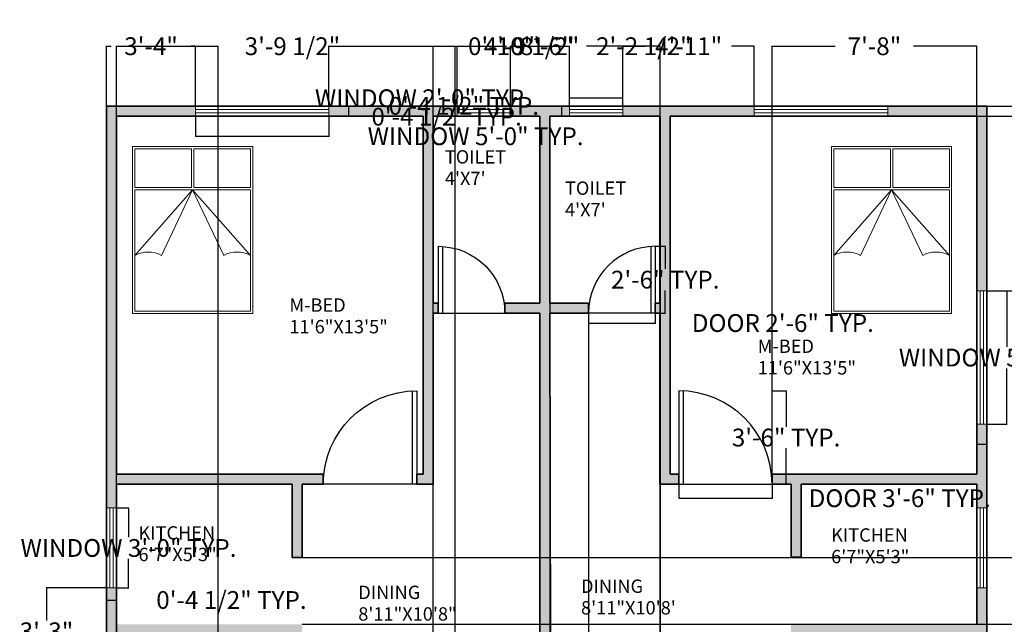
# Model space of a CAD drawing. Units: inches. Extents: x -27 to 662, y -19 to 539.
# Tile 3 of 4: x -18 to 425, y 267 to 539. Entities that reach past the tile are written whole.
import ezdxf

# ---------------------------------------------------------------- set-up
doc = ezdxf.new("R2010")
doc.units = ezdxf.units.IN
doc.header["$MEASUREMENT"] = 0
for name, color, linetype, lineweight in [('A-ANNO-DIMS', 2, 'Continuous', 18), ('A-AREA-IDEN', 230, 'Continuous', 18), ('A-DOOR', 6, 'Continuous', 25), ('A-FURN', 240, 'Continuous', 18), ('A-GLAZ', 240, 'Continuous', 18), ('A-WALL', 4, 'Continuous', 35)]:
    doc.layers.add(name, color=color, linetype=linetype, lineweight=lineweight)
doc.layers.add('A-WALL-PATT', color=2, linetype='Continuous', lineweight=13, true_color=0xf1eb1f)
doc.styles.get("Standard").update_dxf_attribs({"font": 'italic8.shx'})
doc.dimstyles.get("Standard").update_dxf_attribs({"dimtxt": 8, "dimasz": 0.18, "dimexe": 0.18, "dimexo": 0.0625, "dimgap": 0.09, "dimtad": 0, "dimtih": 1, "dimtoh": 1, "dimzin": 0, "dimdsep": 46, "dimlunit": 3, "dimtxsty": 'Standard', "dimcen": 0.09, "dimclrt": 4, "dimadec": 0, "dimazin": 0, "dimtfac": 1, "dimtofl": 0, "dimtmove": 0, "dimatfit": 3, "dimfxl": 1, "dimtolj": 1, "dimtzin": 0, "dimarcsym": 0})

# ---------------------------------------------------------------- blocks, each defined once
blk = doc.blocks.new('*D2')
at = {"layer": 'A-ANNO-DIMS', "color": 0, "lineweight": -2, "transparency": 16777216}
for p, q in [((391.54, 495.42), (467.74, 495.42)), ((467.56, 495.24), (467.56, 262.52)), ((467.56, 20.1), (467.56, 252.82)), ((391.54, 19.92), (467.74, 19.92))]:
    blk.add_line(p, q, dxfattribs=at)
at = {"layer": 'A-ANNO-DIMS', "color": 0, "transparency": 16777216}
for points in [[(467.53, 495.24), (467.59, 495.24), (467.56, 495.42)], [(467.53, 20.1), (467.59, 20.1), (467.56, 19.92)]]:
    blk.add_solid(points, dxfattribs=at)
at = {"layer": 'Defpoints', "color": 0, "transparency": 16777216}
for p in [(391.48, 495.42), (467.56, 495.42), (391.48, 19.92)]:
    blk.add_point(p, dxfattribs=at)
at = {"layer": 'A-ANNO-DIMS', "color": 0, "transparency": 16777216, "insert": (467.56, 257.67), "char_height": 8, "attachment_point": 5}
blk.add_mtext('\\A1;39\'-7.50"', dxfattribs=at)
blk = doc.blocks.new('BED-DOUBLE-54x75')
for p, q in [((26.5, 56.54), (26.5, 74)), ((27.5, 56.54), (27.5, 74)), ((1, 56.54), (26.5, 56.54)), ((1, 55.54), (53, 55.54)), ((27, 55.54), (1, 26.04)), ((13, 26.04), (27, 55.54)), ((27, 55.54), (53, 26.04)), ((41, 26.04), (27, 55.54)), ((27.5, 56.54), (53, 56.54))]:
    blk.add_line(p, q)
blk.add_lwpolyline([(0, 75), (54, 75), (54, 0), (0, 0)], close=True)
for points in [[(1, 56.54), (1, 74), (26.5, 74)], [(27.5, 74), (53, 74), (53, 56.54)], [(53, 55.54), (53, 1), (1, 1), (1, 55.54)]]:
    blk.add_lwpolyline(points)
for centre in [(7, 14.92), (47, 14.92)]:
    blk.add_arc(centre, 12.64, 61.656, 118.344)
blk = doc.blocks.new('DOOR-SWING-30IN')
for p, q in [((28, 29.93), (28, 0)), ((30, 30), (30, 0)), ((30, 0), (0, 0))]:
    blk.add_line(p, q)
blk.add_arc((30, 0), 30, 90, 180)
blk = doc.blocks.new('DOOR-SWING-42IN')
for p, q in [((0, 42), (0, 0)), ((2, 41.95), (2, 0)), ((0, 0), (42, 0))]:
    blk.add_line(p, q)
blk.add_arc((0, 0), 42, 0, 90)
blk = doc.blocks.new('WIN-60IN')
for p, q in [((0, 4.5), (0, 0)), ((60, 4.5), (0, 4.5)), ((60, 0), (60, 4.5)), ((0, 3), (60, 3)), ((0, 1.5), (60, 1.5)), ((0, 0), (60, 0))]:
    blk.add_line(p, q)
blk = doc.blocks.new('WIN-60IN-B')
for p, q in [((0, 0), (0, 60)), ((0, 60), (4.5, 60)), ((1.5, 0), (1.5, 60)), ((3, 0), (3, 60)), ((4.5, 60), (4.5, 0)), ((4.5, 0), (0, 0)), ((4.5, 0), (2.25, 0))]:
    blk.add_line(p, q)
blk = doc.blocks.new('WIN-36IN')
for p, q in [((0, 36), (4.5, 36)), ((0, 0), (0, 36)), ((0, 36), (2.25, 36)), ((1.5, 36), (1.5, 0)), ((3, 36), (3, 0)), ((4.5, 36), (4.5, 0)), ((4.5, 0), (0, 0))]:
    blk.add_line(p, q)
blk = doc.blocks.new('WIN-24IN')
for p, q in [((0, 4.5), (0, 0)), ((24, 4.5), (0, 4.5)), ((24, 0), (24, 4.5)), ((0, 3), (24, 3)), ((0, 1.5), (24, 1.5)), ((0, 0), (24, 0))]:
    blk.add_line(p, q)
blk = doc.blocks.new('*D14')
at = {"layer": 'A-ANNO-DIMS', "color": 0, "lineweight": -2, "transparency": 16777216}
for p, q in [((238.14, 406.86), (238.14, 402.24)), ((268.14, 406.86), (268.14, 402.24)), ((238.32, 402.42), (267.96, 402.42)), ((268.14, 402.42), (268.32, 402.42))]:
    blk.add_line(p, q, dxfattribs=at)
at = {"layer": 'A-ANNO-DIMS', "color": 0, "transparency": 16777216}
for points in [[(238.32, 402.45), (238.32, 402.39), (238.14, 402.42)], [(267.96, 402.45), (267.96, 402.39), (268.14, 402.42)]]:
    blk.add_solid(points, dxfattribs=at)
at = {"layer": 'Defpoints', "color": 0, "transparency": 16777216}
for p in [(238.14, 406.92), (268.14, 406.92), (268.14, 402.42)]:
    blk.add_point(p, dxfattribs=at)
at = {"layer": 'A-ANNO-DIMS', "color": 4, "transparency": 16777216, "insert": (325.55, 402.42), "char_height": 8, "attachment_point": 5}
blk.add_mtext('\\A1;DOOR 2\'-6" TYP.', dxfattribs=at)
blk = doc.blocks.new('*D15')
at = {"layer": 'A-ANNO-DIMS', "color": 0, "lineweight": -2, "transparency": 16777216}
for p, q in [((268.2, 436.92), (272.82, 436.92)), ((272.64, 436.74), (272.64, 426.77)), ((272.64, 407.1), (272.64, 417.07)), ((268.2, 406.92), (272.82, 406.92))]:
    blk.add_line(p, q, dxfattribs=at)
at = {"layer": 'A-ANNO-DIMS', "color": 0, "transparency": 16777216}
for points in [[(272.61, 436.74), (272.67, 436.74), (272.64, 436.92)], [(272.61, 407.1), (272.67, 407.1), (272.64, 406.92)]]:
    blk.add_solid(points, dxfattribs=at)
at = {"layer": 'Defpoints', "color": 0, "transparency": 16777216}
for p in [(268.14, 436.92), (272.64, 436.92), (268.14, 406.92)]:
    blk.add_point(p, dxfattribs=at)
at = {"layer": 'A-ANNO-DIMS', "color": 4, "transparency": 16777216, "insert": (272.64, 421.92), "char_height": 8, "attachment_point": 5}
blk.add_mtext('\\A1;2\'-6" TYP.', dxfattribs=at)
blk = doc.blocks.new('*D16')
at = {"layer": 'A-ANNO-DIMS', "color": 0, "lineweight": -2, "transparency": 16777216}
for p, q in [((278.72, 329.86), (278.72, 323.44)), ((320.72, 329.86), (320.72, 323.44)), ((278.9, 323.62), (320.54, 323.62)), ((320.72, 323.62), (320.9, 323.62))]:
    blk.add_line(p, q, dxfattribs=at)
at = {"layer": 'A-ANNO-DIMS', "color": 0, "transparency": 16777216}
for points in [[(278.9, 323.65), (278.9, 323.59), (278.72, 323.62)], [(320.54, 323.65), (320.54, 323.59), (320.72, 323.62)]]:
    blk.add_solid(points, dxfattribs=at)
at = {"layer": 'Defpoints', "color": 0, "transparency": 16777216}
for p in [(278.72, 329.92), (320.72, 329.92), (320.72, 323.62)]:
    blk.add_point(p, dxfattribs=at)
at = {"layer": 'A-ANNO-DIMS', "color": 4, "transparency": 16777216, "insert": (378.13, 323.62), "char_height": 8, "attachment_point": 5}
blk.add_mtext('\\A1;DOOR 3\'-6" TYP.', dxfattribs=at)
blk = doc.blocks.new('*D17')
at = {"layer": 'A-ANNO-DIMS', "color": 0, "lineweight": -2, "transparency": 16777216}
for p, q in [((320.78, 371.92), (327.2, 371.92)), ((327.02, 371.74), (327.02, 355.77)), ((327.02, 330.1), (327.02, 346.07)), ((320.78, 329.92), (327.2, 329.92))]:
    blk.add_line(p, q, dxfattribs=at)
at = {"layer": 'A-ANNO-DIMS', "color": 0, "transparency": 16777216}
for points in [[(326.99, 371.74), (327.05, 371.74), (327.02, 371.92)], [(326.99, 330.1), (327.05, 330.1), (327.02, 329.92)]]:
    blk.add_solid(points, dxfattribs=at)
at = {"layer": 'Defpoints', "color": 0, "transparency": 16777216}
for p in [(320.72, 371.92), (327.02, 371.92), (320.72, 329.92)]:
    blk.add_point(p, dxfattribs=at)
at = {"layer": 'A-ANNO-DIMS', "color": 4, "transparency": 16777216, "insert": (327.02, 350.92), "char_height": 8, "attachment_point": 5}
blk.add_mtext('\\A1;3\'-6" TYP.', dxfattribs=at)
blk = doc.blocks.new('*D20')
at = {"layer": 'A-ANNO-DIMS', "color": 0, "lineweight": -2, "transparency": 16777216}
for p, q in [((61.34, 495.36), (61.34, 486.24)), ((121.34, 495.36), (121.34, 486.24)), ((61.52, 486.42), (121.16, 486.42)), ((121.34, 486.42), (121.52, 486.42))]:
    blk.add_line(p, q, dxfattribs=at)
at = {"layer": 'A-ANNO-DIMS', "color": 0, "transparency": 16777216}
for points in [[(61.52, 486.45), (61.52, 486.39), (61.34, 486.42)], [(121.16, 486.45), (121.16, 486.39), (121.34, 486.42)]]:
    blk.add_solid(points, dxfattribs=at)
at = {"layer": 'Defpoints', "color": 0, "transparency": 16777216}
for p in [(61.34, 495.42), (121.34, 495.42), (121.34, 486.42)]:
    blk.add_point(p, dxfattribs=at)
at = {"layer": 'A-ANNO-DIMS', "color": 4, "transparency": 16777216, "insert": (187.33, 486.42), "char_height": 8, "attachment_point": 5}
blk.add_mtext('\\A1;WINDOW 5\'-0" TYP.', dxfattribs=at)
blk = doc.blocks.new('*D21')
at = {"layer": 'A-ANNO-DIMS', "color": 0, "lineweight": -2, "transparency": 16777216}
for p, q in [((121.4, 499.92), (130.52, 499.92)), ((130.34, 499.92), (130.34, 500.1)), ((130.34, 500.1), (130.52, 500.1)), ((130.34, 495.6), (130.34, 499.74)), ((121.4, 495.42), (130.52, 495.42))]:
    blk.add_line(p, q, dxfattribs=at)
at = {"layer": 'A-ANNO-DIMS', "color": 0, "transparency": 16777216}
for points in [[(130.31, 499.74), (130.37, 499.74), (130.34, 499.92)], [(130.31, 495.6), (130.37, 495.6), (130.34, 495.42)]]:
    blk.add_solid(points, dxfattribs=at)
at = {"layer": 'Defpoints', "color": 0, "transparency": 16777216}
for p in [(121.34, 499.92), (130.34, 499.92), (121.34, 495.42)]:
    blk.add_point(p, dxfattribs=at)
at = {"layer": 'A-ANNO-DIMS', "color": 4, "transparency": 16777216, "insert": (182.04, 500.1), "char_height": 8, "attachment_point": 5}
blk.add_mtext('\\A1;0\'-4 1/2" TYP.', dxfattribs=at)
blk = doc.blocks.new('*D22')
at = {"layer": 'A-ANNO-DIMS', "color": 0, "lineweight": -2, "transparency": 16777216}
for p, q in [((417.35, 416.88), (426.47, 416.88)), ((426.29, 416.7), (426.29, 391.73)), ((426.29, 357.06), (426.29, 382.03)), ((417.35, 356.88), (426.47, 356.88))]:
    blk.add_line(p, q, dxfattribs=at)
at = {"layer": 'A-ANNO-DIMS', "color": 0, "transparency": 16777216}
for points in [[(426.26, 416.7), (426.32, 416.7), (426.29, 416.88)], [(426.26, 357.06), (426.32, 357.06), (426.29, 356.88)]]:
    blk.add_solid(points, dxfattribs=at)
at = {"layer": 'Defpoints', "color": 0, "transparency": 16777216}
for p in [(417.29, 416.88), (426.29, 416.88), (417.29, 356.88)]:
    blk.add_point(p, dxfattribs=at)
at = {"layer": 'A-ANNO-DIMS', "color": 4, "transparency": 16777216, "insert": (426.29, 386.88), "char_height": 8, "attachment_point": 5}
blk.add_mtext('\\A1;WINDOW 5\'-0" TYP.', dxfattribs=at)
blk = doc.blocks.new('*D23')
at = {"layer": 'A-ANNO-DIMS', "color": 0, "lineweight": -2, "transparency": 16777216}
for p, q in [((412.79, 356.82), (412.79, 347.7)), ((417.29, 356.82), (417.29, 347.7)), ((412.97, 347.88), (417.11, 347.88)), ((417.29, 347.88), (417.47, 347.88))]:
    blk.add_line(p, q, dxfattribs=at)
at = {"layer": 'A-ANNO-DIMS', "color": 0, "transparency": 16777216}
for points in [[(412.97, 347.91), (412.97, 347.85), (412.79, 347.88)], [(417.11, 347.91), (417.11, 347.85), (417.29, 347.88)]]:
    blk.add_solid(points, dxfattribs=at)
at = {"layer": 'Defpoints', "color": 0, "transparency": 16777216}
for p in [(412.79, 356.88), (417.29, 356.88), (417.29, 347.88)]:
    blk.add_point(p, dxfattribs=at)
at = {"layer": 'A-ANNO-DIMS', "color": 4, "transparency": 16777216, "insert": (468.99, 347.88), "char_height": 8, "attachment_point": 5}
blk.add_mtext('\\A1;0\'-4 1/2" TYP.', dxfattribs=at)
blk = doc.blocks.new('*D24')
at = {"layer": 'A-ANNO-DIMS', "color": 0, "lineweight": -2, "transparency": 16777216}
for p, q in [((25.85, 319.25), (31.37, 319.25)), ((31.19, 319.07), (31.19, 306.1)), ((31.19, 283.43), (31.19, 296.4)), ((25.85, 283.25), (31.37, 283.25))]:
    blk.add_line(p, q, dxfattribs=at)
at = {"layer": 'A-ANNO-DIMS', "color": 0, "transparency": 16777216}
for points in [[(31.16, 319.07), (31.22, 319.07), (31.19, 319.25)], [(31.16, 283.43), (31.22, 283.43), (31.19, 283.25)]]:
    blk.add_solid(points, dxfattribs=at)
at = {"layer": 'Defpoints', "color": 0, "transparency": 16777216}
for p in [(25.79, 319.25), (31.19, 319.25), (25.79, 283.25)]:
    blk.add_point(p, dxfattribs=at)
at = {"layer": 'A-ANNO-DIMS', "color": 4, "transparency": 16777216, "insert": (31.19, 301.25), "char_height": 8, "attachment_point": 5}
blk.add_mtext('\\A1;WINDOW 3\'-0" TYP.', dxfattribs=at)
blk = doc.blocks.new('*D25')
at = {"layer": 'A-ANNO-DIMS', "color": 0, "lineweight": -2, "transparency": 16777216}
for p, q in [((21.29, 283.19), (21.29, 277.67)), ((25.79, 283.19), (25.79, 277.67)), ((21.47, 277.85), (25.61, 277.85)), ((25.79, 277.85), (25.97, 277.85))]:
    blk.add_line(p, q, dxfattribs=at)
at = {"layer": 'A-ANNO-DIMS', "color": 0, "transparency": 16777216}
for points in [[(21.47, 277.88), (21.47, 277.82), (21.29, 277.85)], [(25.61, 277.88), (25.61, 277.82), (25.79, 277.85)]]:
    blk.add_solid(points, dxfattribs=at)
at = {"layer": 'Defpoints', "color": 0, "transparency": 16777216}
for p in [(21.29, 283.25), (25.79, 283.25), (25.79, 277.85)]:
    blk.add_point(p, dxfattribs=at)
at = {"layer": 'A-ANNO-DIMS', "color": 4, "transparency": 16777216, "insert": (77.49, 277.85), "char_height": 8, "attachment_point": 5}
blk.add_mtext('\\A1;0\'-4 1/2" TYP.', dxfattribs=at)
blk = doc.blocks.new('*D28')
at = {"layer": 'A-ANNO-DIMS', "color": 0, "lineweight": -2, "transparency": 16777216}
for p, q in [((229.6, 503.52), (229.42, 503.52)), ((229.6, 499.98), (229.6, 503.7)), ((253.42, 503.52), (229.78, 503.52)), ((253.6, 499.98), (253.6, 503.7))]:
    blk.add_line(p, q, dxfattribs=at)
at = {"layer": 'A-ANNO-DIMS', "color": 0, "transparency": 16777216}
for points in [[(229.78, 503.55), (229.78, 503.49), (229.6, 503.52)], [(253.42, 503.55), (253.42, 503.49), (253.6, 503.52)]]:
    blk.add_solid(points, dxfattribs=at)
at = {"layer": 'Defpoints', "color": 0, "transparency": 16777216}
for p in [(229.6, 503.52), (229.6, 499.92), (253.6, 499.92)]:
    blk.add_point(p, dxfattribs=at)
at = {"layer": 'A-ANNO-DIMS', "color": 4, "transparency": 16777216, "insert": (163.62, 503.52), "char_height": 8, "attachment_point": 5}
blk.add_mtext('\\A1;WINDOW 2\'-0" TYP.', dxfattribs=at)
blk = doc.blocks.new('*D29')
at = {"layer": 'A-ANNO-DIMS', "color": 0, "lineweight": -2, "transparency": 16777216}
for p, q in [((229.54, 499.92), (225.82, 499.92)), ((226, 499.74), (226, 495.6)), ((229.54, 495.42), (225.82, 495.42)), ((226, 495.24), (225.82, 495.24)), ((226, 495.42), (226, 495.24))]:
    blk.add_line(p, q, dxfattribs=at)
at = {"layer": 'A-ANNO-DIMS', "color": 0, "transparency": 16777216}
for points in [[(225.97, 499.74), (226.03, 499.74), (226, 499.92)], [(225.97, 495.6), (226.03, 495.6), (226, 495.42)]]:
    blk.add_solid(points, dxfattribs=at)
at = {"layer": 'Defpoints', "color": 0, "transparency": 16777216}
for p in [(229.6, 499.92), (226, 495.42), (229.6, 495.42)]:
    blk.add_point(p, dxfattribs=at)
at = {"layer": 'A-ANNO-DIMS', "color": 4, "transparency": 16777216, "insert": (174.3, 495.24), "char_height": 8, "attachment_point": 5}
blk.add_mtext('\\A1;0\'-4 1/2" TYP.', dxfattribs=at)
blk = doc.blocks.new('*D30')
at = {"layer": 'A-ANNO-DIMS', "color": 0, "lineweight": -2, "transparency": 16777216}
for p, q in [((417.35, 499.92), (444.47, 499.92)), ((444.29, 499.74), (444.29, 264.77)), ((444.29, 20.1), (444.29, 255.07)), ((391.54, 19.92), (444.47, 19.92))]:
    blk.add_line(p, q, dxfattribs=at)
at = {"layer": 'A-ANNO-DIMS', "color": 0, "transparency": 16777216}
for points in [[(444.26, 499.74), (444.32, 499.74), (444.29, 499.92)], [(444.26, 20.1), (444.32, 20.1), (444.29, 19.92)]]:
    blk.add_solid(points, dxfattribs=at)
at = {"layer": 'Defpoints', "color": 0, "transparency": 16777216}
for p in [(417.29, 499.92), (444.29, 499.92), (391.48, 19.92)]:
    blk.add_point(p, dxfattribs=at)
at = {"layer": 'A-ANNO-DIMS', "color": 4, "transparency": 16777216, "insert": (444.29, 259.92), "char_height": 8, "attachment_point": 5}
blk.add_mtext('\\A1;40\'-0"', dxfattribs=at)
blk = doc.blocks.new('*D31')
at = {"layer": 'A-ANNO-DIMS', "color": 0, "lineweight": -2, "transparency": 16777216}
for p, q in [((168.29, 142.48), (168.29, 527.1)), ((168.47, 526.92), (201.29, 526.92)), ((270.11, 526.92), (237.28, 526.92)), ((270.29, 142.48), (270.29, 527.1))]:
    blk.add_line(p, q, dxfattribs=at)
at = {"layer": 'A-ANNO-DIMS', "color": 0, "transparency": 16777216}
for points in [[(168.47, 526.95), (168.47, 526.89), (168.29, 526.92)], [(270.11, 526.95), (270.11, 526.89), (270.29, 526.92)]]:
    blk.add_solid(points, dxfattribs=at)
at = {"layer": 'Defpoints', "color": 0, "transparency": 16777216}
for p in [(270.29, 526.92), (168.29, 142.42), (270.29, 142.42)]:
    blk.add_point(p, dxfattribs=at)
at = {"layer": 'A-ANNO-DIMS', "color": 4, "transparency": 16777216, "insert": (219.29, 526.92), "char_height": 8, "attachment_point": 5}
blk.add_mtext('\\A1;8\'-6"', dxfattribs=at)
blk = doc.blocks.new('*D39')
at = {"layer": 'A-ANNO-DIMS', "color": 0, "lineweight": -2, "transparency": 16777216}
for p, q in [((168.29, 194.98), (168.29, 527.1)), ((168.47, 526.92), (177.98, 526.92)), ((178.16, 194.98), (178.16, 527.1)), ((178.16, 526.92), (178.34, 526.92))]:
    blk.add_line(p, q, dxfattribs=at)
at = {"layer": 'A-ANNO-DIMS', "color": 0, "transparency": 16777216}
for points in [[(168.47, 526.95), (168.47, 526.89), (168.29, 526.92)], [(177.98, 526.95), (177.98, 526.89), (178.16, 526.92)]]:
    blk.add_solid(points, dxfattribs=at)
at = {"layer": 'Defpoints', "color": 0, "transparency": 16777216}
for p in [(178.16, 526.92), (168.29, 194.92), (178.16, 194.92)]:
    blk.add_point(p, dxfattribs=at)
at = {"layer": 'A-ANNO-DIMS', "color": 4, "transparency": 16777216, "insert": (199, 526.92), "char_height": 8, "attachment_point": 5}
blk.add_mtext('\\A1;0\'-10"', dxfattribs=at)
blk = doc.blocks.new('*D41')
at = {"layer": 'A-ANNO-DIMS', "color": 0, "lineweight": -2, "transparency": 16777216}
for p, q in [((21.29, 499.98), (21.29, 527.1)), ((21.47, 526.92), (23.32, 526.92)), ((61.16, 526.92), (59.31, 526.92)), ((61.34, 499.98), (61.34, 527.1))]:
    blk.add_line(p, q, dxfattribs=at)
at = {"layer": 'A-ANNO-DIMS', "color": 0, "transparency": 16777216}
for points in [[(21.47, 526.95), (21.47, 526.89), (21.29, 526.92)], [(61.16, 526.95), (61.16, 526.89), (61.34, 526.92)]]:
    blk.add_solid(points, dxfattribs=at)
at = {"layer": 'Defpoints', "color": 0, "transparency": 16777216}
for p in [(61.34, 526.92), (21.29, 499.92), (61.34, 499.92)]:
    blk.add_point(p, dxfattribs=at)
at = {"layer": 'A-ANNO-DIMS', "color": 4, "transparency": 16777216, "insert": (41.31, 526.92), "char_height": 8, "attachment_point": 5}
blk.add_mtext('\\A1;3\'-4"', dxfattribs=at)
blk = doc.blocks.new('*D42')
at = {"layer": 'A-ANNO-DIMS', "color": 0, "lineweight": -2, "transparency": 16777216}
for p, q in [((121.34, 499.98), (121.34, 527.1)), ((121.52, 526.92), (178.91, 526.92)), ((179.09, 499.98), (179.09, 527.1)), ((179.09, 526.92), (179.27, 526.92))]:
    blk.add_line(p, q, dxfattribs=at)
at = {"layer": 'A-ANNO-DIMS', "color": 0, "transparency": 16777216}
for points in [[(121.52, 526.95), (121.52, 526.89), (121.34, 526.92)], [(178.91, 526.95), (178.91, 526.89), (179.09, 526.92)]]:
    blk.add_solid(points, dxfattribs=at)
at = {"layer": 'Defpoints', "color": 0, "transparency": 16777216}
for p in [(179.09, 526.92), (121.34, 499.92), (179.09, 499.92)]:
    blk.add_point(p, dxfattribs=at)
at = {"layer": 'A-ANNO-DIMS', "color": 4, "transparency": 16777216, "insert": (212.5, 526.92), "char_height": 8, "attachment_point": 5}
blk.add_mtext('\\A1;4\'-9 1/2"', dxfattribs=at)
blk = doc.blocks.new('*D43')
at = {"layer": 'A-ANNO-DIMS', "color": 0, "lineweight": -2, "transparency": 16777216}
for p, q in [((203.09, 499.98), (203.09, 527.1)), ((203.27, 526.92), (229.42, 526.92)), ((229.6, 499.98), (229.6, 527.1)), ((229.6, 526.92), (229.78, 526.92))]:
    blk.add_line(p, q, dxfattribs=at)
at = {"layer": 'A-ANNO-DIMS', "color": 0, "transparency": 16777216}
for points in [[(203.27, 526.95), (203.27, 526.89), (203.09, 526.92)], [(229.42, 526.95), (229.42, 526.89), (229.6, 526.92)]]:
    blk.add_solid(points, dxfattribs=at)
at = {"layer": 'Defpoints', "color": 0, "transparency": 16777216}
for p in [(229.6, 526.92), (203.09, 499.92), (229.6, 499.92)]:
    blk.add_point(p, dxfattribs=at)
at = {"layer": 'A-ANNO-DIMS', "color": 4, "transparency": 16777216, "insert": (263.01, 526.92), "char_height": 8, "attachment_point": 5}
blk.add_mtext('\\A1;2\'-2 1/2"', dxfattribs=at)
blk = doc.blocks.new('*D44')
at = {"layer": 'A-ANNO-DIMS', "color": 0, "lineweight": -2, "transparency": 16777216}
for p, q in [((253.6, 499.98), (253.6, 527.1)), ((253.78, 526.92), (263.83, 526.92)), ((312.54, 526.92), (302.49, 526.92)), ((312.72, 499.98), (312.72, 527.1))]:
    blk.add_line(p, q, dxfattribs=at)
at = {"layer": 'A-ANNO-DIMS', "color": 0, "transparency": 16777216}
for points in [[(253.78, 526.95), (253.78, 526.89), (253.6, 526.92)], [(312.54, 526.95), (312.54, 526.89), (312.72, 526.92)]]:
    blk.add_solid(points, dxfattribs=at)
at = {"layer": 'Defpoints', "color": 0, "transparency": 16777216}
for p in [(312.72, 526.92), (253.6, 499.92), (312.72, 499.92)]:
    blk.add_point(p, dxfattribs=at)
at = {"layer": 'A-ANNO-DIMS', "color": 4, "transparency": 16777216, "insert": (283.16, 526.92), "char_height": 8, "attachment_point": 5}
blk.add_mtext('\\A1;4\'-11"', dxfattribs=at)
blk = doc.blocks.new('*D47')
at = {"layer": 'A-ANNO-DIMS', "color": 0, "lineweight": -2, "transparency": 16777216}
for p, q in [((21.23, 283.25), (-5.89, 283.25)), ((-5.71, 283.07), (-5.71, 268.61)), ((-5.71, 244.45), (-5.71, 258.91)), ((21.23, 244.27), (-5.89, 244.27))]:
    blk.add_line(p, q, dxfattribs=at)
at = {"layer": 'A-ANNO-DIMS', "color": 0, "transparency": 16777216}
for points in [[(-5.74, 283.07), (-5.68, 283.07), (-5.71, 283.25)], [(-5.74, 244.45), (-5.68, 244.45), (-5.71, 244.27)]]:
    blk.add_solid(points, dxfattribs=at)
at = {"layer": 'Defpoints', "color": 0, "transparency": 16777216}
for p in [(-5.71, 283.25), (21.29, 283.25), (21.29, 244.27)]:
    blk.add_point(p, dxfattribs=at)
at = {"layer": 'A-ANNO-DIMS', "color": 4, "transparency": 16777216, "insert": (-5.71, 263.76), "char_height": 8, "attachment_point": 5}
blk.add_mtext('\\A1;3\'-3"', dxfattribs=at)
blk = doc.blocks.new('*D50')
at = {"layer": 'A-ANNO-DIMS', "color": 0, "lineweight": -2, "transparency": 16777216}
for p, q in [((417.35, 499.92), (444.47, 499.92)), ((444.29, 499.74), (444.29, 463.25)), ((444.29, 417.06), (444.29, 453.55)), ((417.35, 416.88), (444.47, 416.88))]:
    blk.add_line(p, q, dxfattribs=at)
at = {"layer": 'A-ANNO-DIMS', "color": 0, "transparency": 16777216}
for points in [[(444.26, 499.74), (444.32, 499.74), (444.29, 499.92)], [(444.26, 417.06), (444.32, 417.06), (444.29, 416.88)]]:
    blk.add_solid(points, dxfattribs=at)
at = {"layer": 'Defpoints', "color": 0, "transparency": 16777216}
for p in [(417.29, 499.92), (444.29, 499.92), (417.29, 416.88)]:
    blk.add_point(p, dxfattribs=at)
at = {"layer": 'A-ANNO-DIMS', "color": 4, "transparency": 16777216, "insert": (444.29, 458.4), "char_height": 8, "attachment_point": 5}
blk.add_mtext('\\A1;6\'-11"', dxfattribs=at)
blk = doc.blocks.new('*D53')
at = {"layer": 'A-ANNO-DIMS', "color": 0, "lineweight": -2, "transparency": 16777216}
for p, q in [((109.35, 296.92), (444.47, 296.92)), ((444.29, 296.74), (444.29, 286.77)), ((444.29, 267.1), (444.29, 277.07)), ((109.35, 266.92), (444.47, 266.92))]:
    blk.add_line(p, q, dxfattribs=at)
at = {"layer": 'A-ANNO-DIMS', "color": 0, "transparency": 16777216}
for points in [[(444.26, 296.74), (444.32, 296.74), (444.29, 296.92)], [(444.26, 267.1), (444.32, 267.1), (444.29, 266.92)]]:
    blk.add_solid(points, dxfattribs=at)
at = {"layer": 'Defpoints', "color": 0, "transparency": 16777216}
for p in [(109.29, 296.92), (444.29, 296.92), (109.29, 266.92)]:
    blk.add_point(p, dxfattribs=at)
at = {"layer": 'A-ANNO-DIMS', "color": 4, "transparency": 16777216, "insert": (444.29, 281.92), "char_height": 8, "attachment_point": 5}
blk.add_mtext('\\A1;2\'-6"', dxfattribs=at)
blk = doc.blocks.new('*D54')
at = {"layer": 'A-ANNO-DIMS', "color": 0, "lineweight": -2, "transparency": 16777216}
for p, q in [((220.8, 406.86), (220.8, -7.26)), ((238.14, 406.86), (238.14, -7.26)), ((220.98, -7.08), (237.96, -7.08)), ((238.14, -7.08), (238.32, -7.08))]:
    blk.add_line(p, q, dxfattribs=at)
at = {"layer": 'A-ANNO-DIMS', "color": 0, "transparency": 16777216}
for points in [[(220.98, -7.05), (220.98, -7.11), (220.8, -7.08)], [(237.96, -7.05), (237.96, -7.11), (238.14, -7.08)]]:
    blk.add_solid(points, dxfattribs=at)
at = {"layer": 'Defpoints', "color": 0, "transparency": 16777216}
for p in [(220.8, 406.92), (238.14, 406.92), (238.14, -7.08)]:
    blk.add_point(p, dxfattribs=at)
at = {"layer": 'A-ANNO-DIMS', "color": 4, "transparency": 16777216, "insert": (270.03, -7.08), "char_height": 8, "attachment_point": 5}
blk.add_mtext('\\A1;1\'-5 1/2"', dxfattribs=at)
blk = doc.blocks.new('*D55')
at = {"layer": 'A-ANNO-DIMS', "color": 0, "lineweight": -2, "transparency": 16777216}
for p, q in [((320.72, 334.48), (320.72, 527.1)), ((320.9, 526.92), (349.14, 526.92)), ((412.61, 526.92), (384.37, 526.92)), ((412.79, 334.48), (412.79, 527.1))]:
    blk.add_line(p, q, dxfattribs=at)
at = {"layer": 'A-ANNO-DIMS', "color": 0, "transparency": 16777216}
for points in [[(320.9, 526.95), (320.9, 526.89), (320.72, 526.92)], [(412.61, 526.95), (412.61, 526.89), (412.79, 526.92)]]:
    blk.add_solid(points, dxfattribs=at)
at = {"layer": 'Defpoints', "color": 0, "transparency": 16777216}
for p in [(412.79, 526.92), (320.72, 334.42), (412.79, 334.42)]:
    blk.add_point(p, dxfattribs=at)
at = {"layer": 'A-ANNO-DIMS', "color": 4, "transparency": 16777216, "insert": (366.75, 526.92), "char_height": 8, "attachment_point": 5}
blk.add_mtext('\\A1;7\'-8"', dxfattribs=at)
blk = doc.blocks.new('*D56')
at = {"layer": 'A-ANNO-DIMS', "color": 0, "lineweight": -2, "transparency": 16777216}
for p, q in [((25.79, 199.48), (25.79, 527.1)), ((25.97, 526.92), (71.34, 526.92)), ((71.52, 199.48), (71.52, 527.1)), ((71.52, 526.92), (71.7, 526.92))]:
    blk.add_line(p, q, dxfattribs=at)
at = {"layer": 'A-ANNO-DIMS', "color": 0, "transparency": 16777216}
for points in [[(25.97, 526.95), (25.97, 526.89), (25.79, 526.92)], [(71.34, 526.95), (71.34, 526.89), (71.52, 526.92)]]:
    blk.add_solid(points, dxfattribs=at)
at = {"layer": 'Defpoints', "color": 0, "transparency": 16777216}
for p in [(71.52, 526.92), (25.79, 199.42), (71.52, 199.42)]:
    blk.add_point(p, dxfattribs=at)
at = {"layer": 'A-ANNO-DIMS', "color": 4, "transparency": 16777216, "insert": (104.93, 526.92), "char_height": 8, "attachment_point": 5}
blk.add_mtext('\\A1;3\'-9 1/2"', dxfattribs=at)
blk = doc.blocks.new('*D58')
at = {"layer": 'A-ANNO-DIMS', "color": 0, "lineweight": -2, "transparency": 16777216}
for p, q in [((220.79, 495.36), (220.79, -7.26)), ((270.29, 495.36), (270.29, -7.26)), ((220.97, -7.08), (270.11, -7.08)), ((270.29, -7.08), (270.47, -7.08))]:
    blk.add_line(p, q, dxfattribs=at)
at = {"layer": 'A-ANNO-DIMS', "color": 0, "transparency": 16777216}
for points in [[(220.97, -7.05), (220.97, -7.11), (220.79, -7.08)], [(270.11, -7.05), (270.11, -7.11), (270.29, -7.08)]]:
    blk.add_solid(points, dxfattribs=at)
at = {"layer": 'Defpoints', "color": 0, "transparency": 16777216}
for p in [(220.79, 495.42), (270.29, 495.42), (270.29, -7.08)]:
    blk.add_point(p, dxfattribs=at)
at = {"layer": 'A-ANNO-DIMS', "color": 4, "transparency": 16777216, "insert": (302.37, -7.08), "char_height": 8, "attachment_point": 5}
blk.add_mtext('\\A1;4\'-1 1/2"', dxfattribs=at)

msp = doc.modelspace()

# ---------------------------------------------------------------- hatches: boundary and pattern name
at = {"layer": 'A-WALL-PATT'}
h = msp.add_hatch(color=256, dxfattribs=at)
h.dxf.hatch_style = 1
h.paths.add_polyline_path([(79.868, 60.419), (25.788, 60.419), (25.788, 105.383), (21.288, 105.383), (21.288, 55.919), (79.868, 55.919)])
h.paths.add_polyline_path([(168.288, 194.919), (178.163, 194.919), (178.163, 199.419), (160.053, 199.419), (160.053, 194.919), (163.788, 194.919), (163.788, 60.419), (139.868, 60.419), (139.868, 58.169), (139.868, 55.919), (163.788, 55.919), (163.788, 19.919), (194.188, 19.919), (194.188, 24.419), (168.288, 24.419)])
h.paths.add_polyline_path([(298.321, 60.419), (274.788, 60.419), (274.788, 194.919), (278.414, 194.919), (278.414, 199.419), (270.288, 199.419), (259.929, 199.419), (259.929, 194.919), (270.288, 194.919), (270.288, 24.419), (242.188, 24.419), (242.188, 19.919), (274.788, 19.919), (274.788, 55.919), (298.321, 55.919)])
h.paths.add_polyline_path([(417.288, 94.965), (412.788, 94.965), (412.788, 60.419), (358.321, 60.419), (358.321, 55.919), (417.288, 55.919)])
h.paths.add_polyline_path([(417.288, 220.271), (412.788, 220.271), (412.788, 199.419), (365.562, 199.419), (365.562, 194.919), (412.788, 194.919), (412.788, 154.965), (417.288, 154.965)])
h.paths.add_polyline_path([(333.788, 262.419), (412.788, 262.419), (412.788, 244.271), (415.038, 244.271), (417.288, 244.271), (417.288, 283.252), (412.788, 283.252), (412.788, 266.919), (329.288, 266.919), (329.288, 262.419), (329.288, 199.419), (320.414, 199.419), (320.414, 194.919), (335.562, 194.919), (335.562, 199.419), (333.788, 199.419)])
h.paths.add_polyline_path([(333.788, 329.919), (412.788, 329.919), (412.788, 319.252), (415.038, 319.252), (417.288, 319.252), (417.288, 356.883), (415.038, 356.883), (412.788, 356.883), (412.788, 334.419), (320.72, 334.419), (320.72, 329.919), (329.288, 329.919), (329.288, 297.07), (333.788, 297.07)])
h.paths.add_polyline_path([(220.796, 406.919), (238.139, 406.919), (238.139, 411.419), (220.788, 411.419), (220.788, 495.419), (229.602, 495.419), (229.602, 499.919), (203.089, 499.919), (203.089, 495.419), (216.288, 495.419), (216.288, 411.419), (200.507, 411.419), (200.507, 406.919), (216.288, 406.919), (216.288, 199.419), (214.163, 199.419), (214.163, 194.919), (223.929, 194.919), (223.929, 199.419), (221.182, 199.419)])
h.paths.add_polyline_path([(109.288, 266.919), (104.788, 266.919), (25.788, 266.919), (25.788, 262.419), (104.788, 262.419), (104.788, 199.419), (101.522, 199.419), (101.522, 194.919), (118.053, 194.919), (118.053, 199.419), (109.288, 199.419)])
h.paths.add_polyline_path([(71.522, 199.419), (25.788, 199.419), (25.788, 220.271), (21.288, 220.271), (21.288, 165.383), (25.788, 165.383), (25.788, 194.919), (71.522, 194.919)])
h.paths.add_polyline_path([(25.788, 283.252), (21.288, 283.252), (21.288, 244.271), (23.538, 244.271), (25.788, 244.271)])
h.paths.add_polyline_path([(118.822, 334.419), (25.788, 334.419), (25.788, 495.419), (61.341, 495.419), (61.341, 499.919), (21.288, 499.919), (21.288, 319.252), (23.538, 319.252), (25.788, 319.252), (25.788, 329.919), (104.788, 329.919), (104.788, 296.919), (109.288, 296.919), (109.288, 329.919), (118.822, 329.919)])
h.paths.add_polyline_path([(168.288, 406.919), (170.507, 406.919), (170.507, 411.419), (168.288, 411.419), (168.288, 495.419), (179.089, 495.419), (179.089, 499.919), (121.341, 499.919), (121.341, 495.419), (163.788, 495.419), (163.788, 334.419), (160.822, 334.419), (160.822, 329.919), (168.288, 329.919)])
h.paths.add_polyline_path([(312.716, 499.919), (253.602, 499.919), (253.602, 495.419), (270.288, 495.419), (270.288, 411.419), (268.139, 411.419), (268.139, 406.919), (270.288, 406.919), (270.288, 329.919), (278.72, 329.919), (278.72, 334.419), (274.788, 334.419), (274.788, 495.419), (312.716, 495.419)])
h.paths.add_polyline_path([(417.288, 499.919), (372.716, 499.919), (372.716, 495.419), (412.788, 495.419), (412.788, 416.883), (417.288, 416.883)])

# ---------------------------------------------------------------- linework, layer by layer
at = {"layer": 'A-WALL'}
for p, q in [((417.288, 499.919), (21.288, 499.919)), ((21.288, 499.919), (21.288, 55.919)), ((417.288, 55.919), (417.288, 499.919)), ((25.788, 495.419), (25.788, 334.419)), ((163.788, 495.419), (25.788, 495.419)), ((163.788, 495.419), (163.788, 334.419)), ((168.288, 495.419), (168.288, 411.419)), ((216.288, 495.419), (168.288, 495.419)), ((216.288, 495.419), (216.288, 411.419)), ((270.288, 495.419), (220.788, 495.419)), ((220.788, 495.419), (220.788, 411.419)), ((270.288, 411.419), (270.288, 495.419)), ((412.788, 495.419), (274.788, 495.419)), ((274.788, 334.419), (274.788, 495.419)), ((412.788, 334.419), (412.788, 495.419)), ((170.507, 411.419), (168.288, 411.419)), ((170.507, 411.419), (170.507, 406.919)), ((216.288, 411.419), (200.507, 411.419)), ((200.507, 411.419), (200.507, 406.919)), ((238.139, 411.419), (220.788, 411.419)), ((238.139, 406.919), (238.139, 411.419)), ((270.288, 411.419), (268.139, 411.419)), ((268.139, 406.919), (268.139, 411.419)), ((168.288, 406.919), (168.288, 329.919)), ((170.507, 406.919), (168.288, 406.919)), ((216.288, 406.919), (200.507, 406.919)), ((216.288, 406.919), (216.288, 199.419)), ((220.796, 406.919), (221.182, 199.419)), ((238.139, 406.919), (220.796, 406.919)), ((270.288, 406.919), (268.139, 406.919)), ((270.288, 329.919), (270.288, 406.919)), ((118.822, 334.419), (25.788, 334.419)), ((118.822, 334.419), (118.822, 329.919)), ((163.788, 334.419), (160.822, 334.419)), ((160.822, 334.419), (160.822, 329.919)), ((278.72, 334.419), (274.788, 334.419)), ((278.72, 334.419), (278.72, 329.919)), ((412.788, 334.419), (320.72, 334.419)), ((320.72, 334.419), (320.72, 329.919)), ((25.788, 329.919), (25.788, 199.419)), ((104.788, 329.919), (25.788, 329.919)), ((104.788, 329.919), (104.788, 296.919)), ((109.288, 329.919), (109.288, 296.919)), ((118.822, 329.919), (109.288, 329.919)), ((168.288, 329.919), (160.822, 329.919)), ((278.72, 329.919), (270.288, 329.919)), ((329.288, 329.919), (320.72, 329.919)), ((329.288, 297.07), (329.288, 329.919)), ((412.788, 329.919), (333.788, 329.919)), ((333.788, 297.07), (333.788, 329.919)), ((412.788, 266.919), (412.788, 329.919)), ((104.788, 296.919), (109.288, 296.919)), ((329.288, 297.07), (333.788, 297.07))]:
    msp.add_line(p, q, dxfattribs=at)

# ---------------------------------------------------------------- block references
at = {"layer": 'A-DOOR', "extrusion": (0, 0, -1), "zscale": -1}
for name, p in [('DOOR-SWING-30IN', (-200.507, 406.919)), ('DOOR-SWING-42IN', (-160.821, 329.919))]:
    msp.add_blockref(name, p, dxfattribs=at)
at = {"layer": 'A-DOOR'}
for name, p in [('DOOR-SWING-30IN', (238.139, 406.919)), ('DOOR-SWING-42IN', (278.72, 329.919))]:
    msp.add_blockref(name, p, dxfattribs=at)
at = {"layer": 'A-FURN'}
for p in [(33.046, 406.772), (347.468, 406.772)]:
    msp.add_blockref('BED-DOUBLE-54x75', p, dxfattribs=at)
at = {"layer": 'A-GLAZ'}
for name, p in [('WIN-60IN', (61.341, 495.419)), ('WIN-24IN', (179.089, 495.419)), ('WIN-60IN-B', (412.788, 356.883)), ('WIN-36IN', (21.288, 283.252)), ('WIN-36IN', (412.788, 283.252))]:
    msp.add_blockref(name, p, dxfattribs=at)
at = {"layer": 'A-GLAZ', "rotation": 180}
for name, p in [('WIN-24IN', (253.602, 499.92)), ('WIN-60IN', (372.717, 499.92))]:
    msp.add_blockref(name, p, dxfattribs=at)

# ---------------------------------------------------------------- texts
at = {"layer": 'A-AREA-IDEN'}
for s, p in [('TOILET', (173.509, 474.166)), ("4'X7'", (173.509, 464.452)), ('TOILET', (227.547, 460.091)), ("4'X7'", (227.547, 450.376)), ('M-BED', (103.581, 407.496)), ('11\'6"X13\'5"', (103.581, 397.782)), ('M-BED', (314.229, 388.988)), ('11\'6"X13\'5"', (314.229, 379.273)), ('KITCHEN', (35.666, 305.048)), ('KITCHEN', (347.279, 304.093)), ('6\'7"X5\'3"', (35.666, 295.334)), ('6\'7"X5\'3"', (347.279, 294.378)), ('DINING', (134.55, 278.291)), ('DINING', (234.766, 281.055)), ('8\'11"X10\'8"', (134.55, 268.577)), ('8\'11"X10\'8\'', (234.766, 271.341))]:
    msp.add_text(s, height=6, dxfattribs=at).set_placement(p)

# ---------------------------------------------------------------- dimensions: what is measured, and where the dimension line sits
at = {"layer": 'A-ANNO-DIMS'}
for base, p1, p2, picture, middle in [((71.522, 526.919), (25.788, 199.419), (71.522, 199.419), '*D56', (104.935, 526.919)), ((179.089, 526.919), (121.341, 499.919), (179.089, 499.919), '*D42', (212.502, 526.919)), ((229.602, 526.919), (203.089, 499.919), (229.602, 499.919), '*D43', (263.015, 526.919)), ((61.341, 526.919), (21.288, 499.919), (61.341, 499.919), '*D41', (41.315, 526.919)), ((270.288, 526.919), (168.288, 142.419), (270.288, 142.419), '*D31', (219.288, 526.919)), ((178.163, 526.919), (168.288, 194.919), (178.163, 194.919), '*D39', (199.004, 526.919)), ((312.716, 526.919), (253.602, 499.919), (312.716, 499.919), '*D44', (283.159, 526.919)), ((412.788, 526.919), (320.72, 334.419), (412.788, 334.419), '*D55', (366.754, 526.919)), ((270.288, -7.081), (220.788, 495.419), (270.288, 495.419), '*D58', (302.367, -7.081)), ((238.139, -7.081), (220.796, 406.919), (238.139, 406.919), '*D54', (270.028, -7.081))]:
    dim = msp.add_linear_dim(base=base, p1=p1, p2=p2, dimstyle='Standard', override={"dimdec": 1, "dimlfac": 1, "dimrnd": 0, "dimzin": 1, "dimdsep": 46, "dimlunit": 4, "dimfrac": 2}, dxfattribs=at)
    dim.commit()
    dim.dimension.update_dxf_attribs({"geometry": picture, "text_midpoint": middle})
for base, p1, p2, angle, text, picture, middle in [((229.602, 503.519), (253.602, 499.919), (229.602, 499.919), 180, 'WINDOW <> TYP.', '*D28', (163.617, 503.519)), ((130.341, 499.919), (121.341, 495.419), (121.341, 499.919), 90, '<> TYP.', '*D21', (182.04, 500.099)), ((226.002, 495.419), (229.602, 499.919), (229.602, 495.419), 270, '<> TYP.', '*D29', (174.303, 495.239)), ((272.639, 436.919), (268.139, 406.919), (268.139, 436.919), 90, '<> TYP.', '*D15', (272.639, 421.919)), ((426.288, 416.883), (417.288, 356.883), (417.288, 416.883), 90, 'WINDOW <> TYP.', '*D22', (426.288, 386.883)), ((327.02, 371.919), (320.72, 329.919), (320.72, 371.919), 90, '<> TYP.', '*D17', (327.02, 350.919)), ((31.188, 319.252), (25.788, 283.252), (25.788, 319.252), 90, 'WINDOW <> TYP.', '*D24', (31.188, 301.252))]:
    dim = msp.add_linear_dim(base=base, p1=p1, p2=p2, angle=angle, text=text, dimstyle='Standard', override={"dimdec": 1, "dimlfac": 1, "dimrnd": 0, "dimzin": 1, "dimdsep": 46, "dimlunit": 4, "dimfrac": 2}, dxfattribs=at)
    dim.commit()
    dim.dimension.update_dxf_attribs({"geometry": picture, "text_midpoint": middle})
for base, p1, p2, text, picture, middle in [((121.341, 486.419), (61.341, 495.419), (121.341, 495.419), 'WINDOW <> TYP.', '*D20', (187.326, 486.419)), ((268.139, 402.419), (238.139, 406.919), (268.139, 406.919), 'DOOR <> TYP.', '*D14', (325.552, 402.419)), ((417.288, 347.883), (412.788, 356.883), (417.288, 356.883), '<> TYP.', '*D23', (468.986, 347.883)), ((320.72, 323.619), (278.72, 329.919), (320.72, 329.919), 'DOOR <> TYP.', '*D16', (378.133, 323.619)), ((25.788, 277.852), (21.288, 283.252), (25.788, 283.252), '<> TYP.', '*D25', (77.486, 277.852))]:
    dim = msp.add_linear_dim(base=base, p1=p1, p2=p2, text=text, dimstyle='Standard', override={"dimdec": 1, "dimlfac": 1, "dimrnd": 0, "dimzin": 1, "dimdsep": 46, "dimlunit": 4, "dimfrac": 2}, dxfattribs=at)
    dim.commit()
    dim.dimension.update_dxf_attribs({"geometry": picture, "text_midpoint": middle})
for base, p1, p2, override, picture, middle in [((444.288, 499.919), (391.48, 19.919), (417.288, 499.919), {"dimdec": 1, "dimlfac": 1, "dimrnd": 0, "dimzin": 1, "dimdsep": 46, "dimlunit": 4, "dimfrac": 2}, '*D30', (444.288, 259.919)), ((444.288, 499.919), (417.288, 416.883), (417.288, 499.919), {"dimdec": 1, "dimlfac": 1, "dimrnd": 0, "dimzin": 1, "dimdsep": 46, "dimlunit": 4, "dimfrac": 2}, '*D50', (444.288, 458.401)), ((467.557, 495.419), (391.48, 19.919), (391.48, 495.419), {"dimclrd": 0, "dimclre": 0, "dimclrt": 0}, '*D2', (467.557, 257.669)), ((444.288, 296.919), (109.288, 266.919), (109.288, 296.919), {"dimdec": 1, "dimlfac": 1, "dimrnd": 0, "dimzin": 1, "dimdsep": 46, "dimlunit": 4, "dimfrac": 2}, '*D53', (444.288, 281.919)), ((-5.712, 283.252), (21.288, 244.271), (21.288, 283.252), {"dimdec": 1, "dimlfac": 1, "dimrnd": 0, "dimzin": 1, "dimdsep": 46, "dimlunit": 4, "dimfrac": 2}, '*D47', (-5.712, 263.762))]:
    dim = msp.add_linear_dim(base=base, p1=p1, p2=p2, angle=90, dimstyle='Standard', override=override, dxfattribs=at)
    dim.commit()
    dim.dimension.update_dxf_attribs({"geometry": picture, "text_midpoint": middle})

doc.saveas('drawing.dxf')
